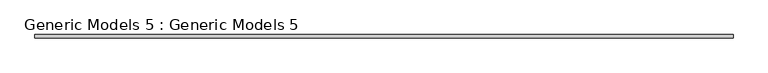
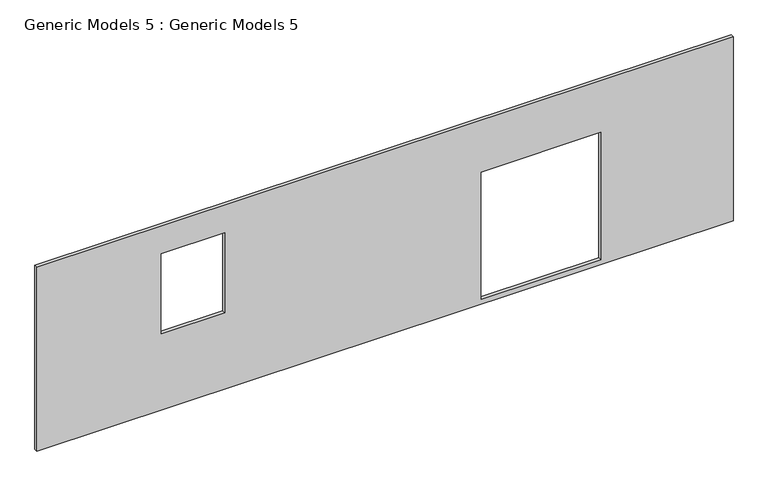
"""IFC4 building model written with IfcOpenShell, lengths in millimetres: proxy geometry, Generic Models 5 : Generic Models 5."""

from ifc_helpers import new_model, si_unit, frame, origin, place, context, project, spatial, polyline, outline, extrude, source, transform, mapped, element, save


def generic_models_5_generic_models_5_2da6e60e(model_context):
    return source(origin(), model_context, "Body", "SweptSolid", [
        extrude(outline(polyline([(9324.8120259, -6097.4280307), (6520.0580357, -6097.4280307), (6520.0580357, 3960.9719693), (9324.8120259, 3960.9719693), (9324.8120259, -6097.4280307)]), holes=[polyline([(8534.4, 2049.6219693), (6592.1705726, 2049.6219693), (6592.1705726, 322.4219693), (8534.4, 322.4219693), (8534.4, 2049.6219693)]), polyline([(8904.9782243, -3385.9780307), (7685.7782243, -3385.9780307), (7685.7782243, -4300.3780307), (8904.9782243, -4300.3780307), (8904.9782243, -3385.9780307)])]), frame((0.0, 1676.4641252, 0.0), z_axis=(0.0, 1.0, 0.0), x_axis=(0.0, 0.0, 1.0)), (0.0, 0.0, 1.0), 50.8),
    ])


if __name__ == "__main__":
    model = new_model("IFC4")
    model_context = context("Model", 3, world=origin())
    ifc_project = project(units=[si_unit("LENGTHUNIT", "METRE", prefix="MILLI")], contexts=[model_context])
    site = spatial("IfcSite", under=ifc_project)
    building = spatial("IfcBuilding", under=site)
    placement = place(None, origin())
    generic_models_5_generic_models_5_shape = generic_models_5_generic_models_5_2da6e60e(model_context)
    element("IfcBuildingElementProxy", 1, Name="Generic Models 5 : Generic Models 5", ObjectType="Generic Models 5 : Generic Models 5", at=placement, inside=building, context=model_context, shape_type="MappedRepresentation", body=[
        mapped(generic_models_5_generic_models_5_shape, transform((0.0, 0.0, 0.0), x_axis=(1.0, 0.0, 0.0), y_axis=(0.0, 1.0, 0.0), z_axis=(0.0, 0.0, 1.0))),
    ])
    save(model, "model.ifc")
